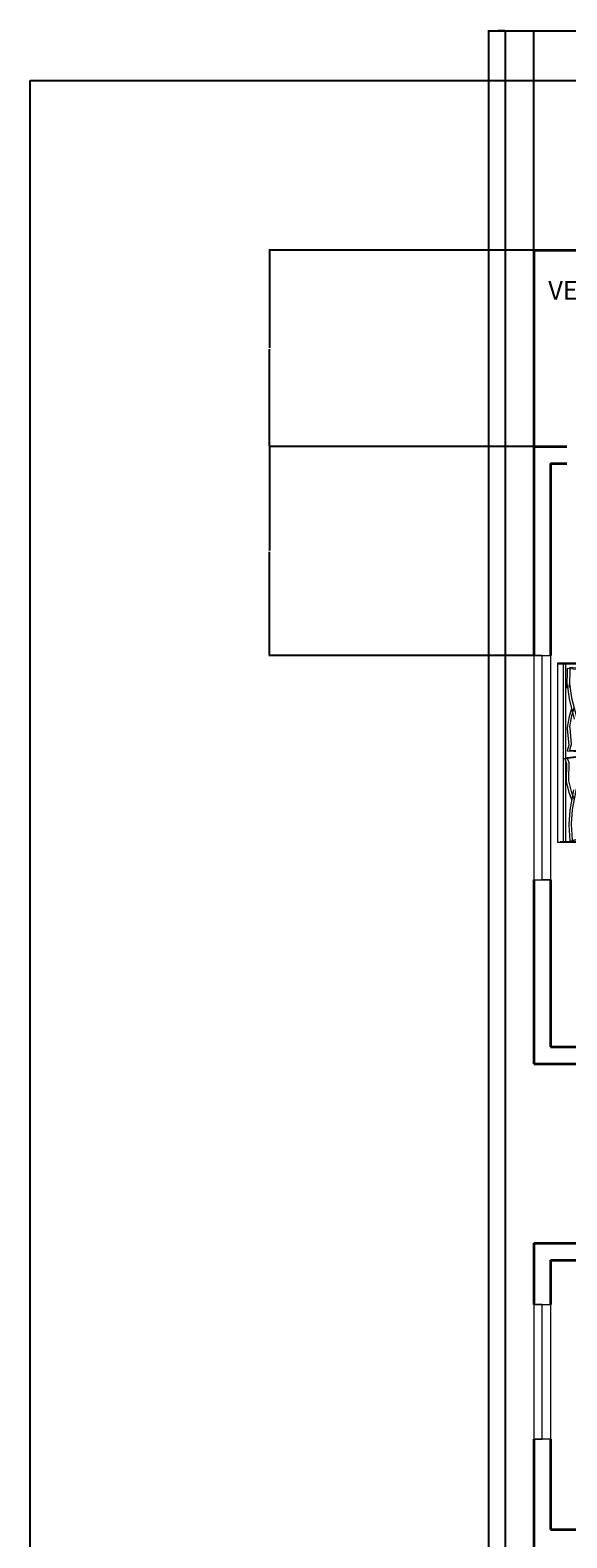
# Model space of a CAD drawing. Units: inches. Extents: x 2163 to 2982, y 1024 to 2288.
# Tile 10 of 22: x 2163 to 2306, y 1885 to 2288. Entities that reach past the tile are written whole.
import ezdxf

# ---------------------------------------------------------------- set-up
doc = ezdxf.new("R2010")
doc.units = ezdxf.units.IN
for name, color, linetype, lineweight in [('A-ANNO-DIMS', 2, 'Continuous', 18), ('A-ANNO-TTLB', 7, 'Continuous', 25), ('A-AREA-IDEN', 7, 'Continuous', 18), ('A-FURN', 8, 'Continuous', 13), ('A-GLAZ', 161, 'Continuous', 18), ('A-WALL', 7, 'Continuous', 35)]:
    doc.layers.add(name, color=color, linetype=linetype, lineweight=lineweight)
doc.styles.get("Standard").update_dxf_attribs({"font": 'arial.ttf'})
doc.dimstyles.get("Standard").update_dxf_attribs({"dimtxt": 0.18, "dimasz": 0.18, "dimexe": 0.18, "dimexo": 0.0625, "dimgap": 0.09, "dimtad": 0, "dimtih": 1, "dimtoh": 1, "dimdec": 4, "dimzin": 0, "dimdsep": 46, "dimtxsty": 'Standard', "dimcen": 0.09, "dimadec": 0, "dimazin": 0, "dimtfac": 1, "dimtdec": 4, "dimtofl": 0, "dimtmove": 0, "dimatfit": 3, "dimfxl": 1, "dimtolj": 1, "dimtzin": 0, "dimarcsym": 0})

# ---------------------------------------------------------------- blocks, each defined once
blk = doc.blocks.new('BED-DOUBLE')
for p, q in [((27.75, 52.87), (24.5, 49.16)), ((27.75, 52.87), (24.5, 49.16)), ((28.38, 53.1), (25.13, 49.39)), ((28.38, 53.1), (25.13, 49.39)), ((29.49, 52.95), (27.75, 52.87, 3.87)), ((29.49, 52.95), (27.75, 52.87, 3.87)), ((28.36, 51.33), (27.75, 52.87)), ((28.36, 51.33), (27.75, 52.87)), ((30.13, 53.18), (28.38, 53.1, 3.87)), ((29, 51.56), (28.38, 53.1)), ((30.13, 53.18), (28.38, 53.1, 3.87)), ((29, 51.56), (28.38, 53.1)), ((0, 51.49), (0.64, 51.49)), ((0, 3.47), (0, 51.49)), ((0, 51.27), (26.61, 51.27)), ((0, 51.27), (26.61, 51.27)), ((0.64, 51.49), (27.25, 51.49)), ((0.64, 51.49), (27.25, 51.49)), ((1.53, 3.48), (1.53, 51.27)), ((1.53, 3.47), (1.53, 51.27)), ((2.17, 3.7), (2.17, 51.49)), ((2.17, 3.7), (2.17, 51.49)), ((2.56, 50.11), (2.46, 44.71)), ((2.56, 50.11), (2.46, 44.71)), ((2.56, 50.11), (5.77, 49.73)), ((2.56, 50.11), (5.77, 49.73)), ((3.2, 50.34), (3.1, 44.94)), ((3.2, 50.34), (3.1, 44.94)), ((3.2, 50.34), (6.41, 49.96)), ((3.2, 50.34), (6.41, 49.96)), ((8.26, 49.31), (5.58, 48.13)), ((8.26, 49.31), (5.58, 48.13)), ((5.77, 49.73), (8.34, 50.33)), ((5.77, 49.73), (8.34, 50.33)), ((8.9, 49.54), (6.22, 48.36)), ((8.9, 49.54), (6.22, 48.36)), ((6.41, 49.96), (8.98, 50.56)), ((6.41, 49.96), (8.98, 50.56)), ((11.83, 50.11), (8.26, 49.31)), ((11.83, 50.11), (8.26, 49.31)), ((8.34, 50.33), (9.38, 49.81)), ((8.34, 50.33), (9.38, 49.81)), ((12.47, 50.34), (8.9, 49.54)), ((12.47, 50.34), (8.9, 49.54)), ((8.98, 50.56), (10.02, 50.04)), ((8.98, 50.56), (10.02, 50.04)), ((13.43, 49.92), (11.83, 50.11)), ((13.43, 49.92), (11.83, 50.11)), ((14.07, 50.15), (12.47, 50.34)), ((14.07, 50.15), (12.47, 50.34)), ((16.57, 50.7), (13.43, 49.92)), ((16.57, 50.7), (13.43, 49.92)), ((17.21, 50.93), (14.07, 50.15)), ((17.21, 50.93), (14.07, 50.15)), ((16.17, 45.57), (16.57, 50.7)), ((16.17, 45.57), (16.57, 50.7)), ((16.81, 45.79), (17.21, 50.93)), ((16.81, 45.79), (17.21, 50.93)), ((24.5, 49.16), (22.33, 46.22)), ((24.5, 49.16), (22.33, 46.22)), ((25.13, 49.39), (22.97, 46.45)), ((25.13, 49.39), (22.97, 46.45)), ((28.06, 48.23), (28.36, 51.33)), ((28.06, 48.23), (28.36, 51.33)), ((28.69, 48.46), (29, 51.56)), ((28.69, 48.46), (29, 51.56)), ((29, 44.59), (28.69, 48.46)), ((29, 44.59), (28.69, 48.46)), ((2.46, 44.71), (2.54, 45.71)), ((2.46, 44.71), (2.54, 45.71)), ((2.54, 45.71), (3.07, 41.91)), ((2.54, 45.71), (3.07, 41.91)), ((3.1, 44.94), (3.18, 45.94)), ((3.1, 44.94), (3.18, 45.94)), ((3.18, 45.94), (3.71, 42.14)), ((3.18, 45.94), (3.71, 42.14)), ((16.73, 43.61), (16.17, 45.57)), ((16.73, 43.61), (16.17, 45.57)), ((17.37, 43.83), (16.81, 45.79)), ((17.37, 43.83), (16.81, 45.79)), ((22.33, 46.22), (20.32, 40.64)), ((22.33, 46.22), (20.32, 40.64)), ((22.97, 46.45), (20.96, 40.87)), ((22.97, 46.45), (20.96, 40.87)), ((28.36, 44.36), (28.06, 48.23)), ((28.36, 44.36), (28.06, 48.23)), ((28.83, 40.95), (28.36, 44.36)), ((28.83, 40.95), (28.36, 44.36)), ((29.47, 41.18), (29, 44.59)), ((29.47, 41.18), (29, 44.59)), ((3.07, 41.91), (4.42, 36.49)), ((3.07, 41.91), (4.42, 36.49)), ((3.71, 42.14), (5.06, 36.72)), ((3.71, 42.14), (5.06, 36.72)), ((16.29, 36.6), (16.73, 43.61)), ((16.29, 36.6), (16.73, 43.61)), ((16.93, 36.82), (17.37, 43.83)), ((16.93, 36.82), (17.37, 43.83)), ((20.32, 40.64), (17.38, 32.31)), ((20.32, 40.64), (17.38, 32.31)), ((20.96, 40.87), (18.02, 32.53)), ((20.96, 40.87), (18.02, 32.53)), ((29.76, 38.94), (28.83, 40.95)), ((29.76, 38.94), (28.83, 40.95)), ((30.4, 39.17), (29.47, 41.18)), ((30.4, 39.17), (29.47, 41.18)), ((3.08, 37.14), (2.54, 34.2)), ((3.08, 37.13), (2.54, 34.2)), ((3.67, 39.2), (3.08, 37.14)), ((3.67, 39.2), (3.08, 37.13)), ((3.72, 37.36), (3.18, 34.43)), ((3.72, 37.36), (3.18, 34.43)), ((4.31, 39.43), (3.72, 37.36)), ((4.31, 39.43), (3.72, 37.36)), ((15.63, 32.56), (16.29, 36.6)), ((15.63, 32.56), (16.29, 36.6)), ((16.27, 32.79), (16.93, 36.82)), ((16.27, 32.79), (16.93, 36.82)), ((24.52, 34.68), (29, 36.38)), ((24.52, 34.68), (29, 36.38)), ((28.36, 36.15), (30.38, 36.46)), ((28.36, 36.15), (30.38, 36.46)), ((29, 36.38), (31.02, 36.69)), ((29, 36.38), (31.02, 36.69)), ((30.38, 36.46), (29.76, 38.94)), ((30.38, 36.46), (29.76, 38.94)), ((31.02, 36.69), (30.4, 39.17)), ((31.02, 36.69), (30.4, 39.17)), ((79.24, 15.06), (79.24, 39.68)), ((79.24, 15.06), (79.24, 39.68)), ((79.88, 15.29), (79.88, 39.91)), ((79.88, 15.29), (79.88, 39.91)), ((2.54, 34.2), (2.56, 33.88)), ((2.54, 34.2), (2.56, 33.88)), ((2.56, 33.88), (2.98, 29.46)), ((2.56, 33.88), (2.98, 29.46)), ((3.18, 34.43), (3.2, 34.11)), ((3.18, 34.43), (3.2, 34.11)), ((3.2, 34.11), (3.62, 29.68)), ((3.2, 34.11), (3.62, 29.68)), ((16.74, 30.75), (15.45, 33.82)), ((16.74, 30.75), (15.45, 33.82)), ((17.38, 30.98), (16.09, 34.05)), ((17.38, 30.98), (16.09, 34.05)), ((17.38, 30.26), (23.88, 34.45)), ((17.38, 30.26), (23.88, 34.45)), ((18.02, 30.49), (24.52, 34.68)), ((18.02, 30.49), (24.52, 34.68)), ((23.88, 34.45), (28.36, 36.15)), ((23.88, 34.45), (28.36, 36.15)), ((2.98, 29.46), (2.49, 27.98)), ((2.98, 29.46), (2.49, 27.98)), ((3.62, 29.68), (3.13, 28.21)), ((3.62, 29.68), (3.13, 28.2)), ((13.02, 27.66), (14.86, 28.36)), ((13.02, 27.66), (14.86, 28.36)), ((14.22, 28.13), (16.89, 28.3)), ((14.22, 28.13), (16.89, 28.3)), ((14.86, 28.36), (17.53, 28.53)), ((14.86, 28.36), (17.53, 28.53)), ((16.89, 28.3), (16.74, 30.75)), ((16.89, 28.3), (16.74, 30.75)), ((17.53, 28.53), (17.38, 30.98)), ((17.53, 28.53), (17.38, 30.98)), ((1.87, 25.98), (7.22, 26.56)), ((1.87, 25.98), (7.22, 26.56)), ((2.45, 24.54), (1.87, 25.98)), ((2.45, 24.54), (1.87, 25.98)), ((2.3, 20.09), (2.45, 24.54)), ((2.3, 20.09), (2.45, 24.54)), ((2.49, 27.98), (7.87, 27.73)), ((2.49, 27.98), (7.87, 27.73)), ((2.51, 26.21), (7.86, 26.79)), ((2.51, 26.21), (7.86, 26.79)), ((3.09, 24.77), (2.51, 26.21)), ((3.09, 24.77), (2.51, 26.21)), ((2.94, 20.32), (3.09, 24.77)), ((2.94, 20.32), (3.09, 24.77)), ((3.13, 28.21), (8.51, 27.96)), ((3.13, 28.2), (8.51, 27.96)), ((7.22, 26.56), (10.4, 27.14)), ((7.22, 26.56), (10.4, 27.14)), ((7.86, 26.79), (11.04, 27.37)), ((7.86, 26.79), (11.04, 27.37)), ((7.87, 27.73), (11.08, 27.35)), ((7.87, 27.73), (11.08, 27.35)), ((8.51, 27.96), (11.72, 27.58)), ((8.51, 27.96), (11.72, 27.58)), ((10.4, 27.14), (11.7, 27.14)), ((10.4, 27.14), (11.7, 27.14)), ((11.04, 27.37), (12.34, 27.37)), ((11.04, 27.37), (12.34, 27.37)), ((11.08, 27.35), (12.38, 27.44)), ((11.08, 27.35), (12.38, 27.44)), ((11.7, 27.14), (13.58, 26.56)), ((11.7, 27.14), (13.58, 26.56)), ((11.72, 27.58), (13.02, 27.66)), ((11.72, 27.58), (13.02, 27.66)), ((12.34, 27.37), (14.22, 26.79)), ((12.34, 27.37), (14.22, 26.79)), ((12.38, 27.44), (14.22, 28.13)), ((12.38, 27.44), (14.22, 28.13)), ((13.58, 26.56), (16.26, 26.56)), ((13.58, 26.56), (16.26, 26.56)), ((14.22, 26.79), (16.9, 26.79)), ((14.22, 26.79), (16.9, 26.79)), ((16.9, 24.33), (15.81, 21.19)), ((16.9, 24.33), (15.81, 21.19)), ((16.17, 19.38), (16.57, 24.52)), ((16.17, 19.38), (16.57, 24.52)), ((16.26, 26.56), (16.26, 24.1)), ((16.26, 26.56), (16.26, 24.1)), ((16.81, 19.61), (17.21, 24.74)), ((16.81, 19.61), (17.21, 24.74)), ((16.9, 26.79), (16.9, 24.33)), ((16.9, 26.79), (16.9, 24.33)), ((2.94, 20), (2.94, 20.32)), ((2.94, 20), (2.94, 20.32)), ((16.26, 24.1), (15.17, 20.96)), ((16.26, 24.1), (15.17, 20.96)), ((2.3, 19.77), (2.3, 20.09)), ((2.3, 19.77), (2.3, 20.09)), ((3.03, 16.88), (2.3, 19.77)), ((3.03, 16.88), (2.3, 19.77)), ((3.67, 17.11), (2.94, 20)), ((3.67, 17.11), (2.94, 20)), ((3.75, 14.85), (3.03, 16.88)), ((3.75, 14.85), (3.03, 16.88)), ((3.32, 12.11), (4.33, 17.6)), ((3.32, 12.11), (4.33, 17.6)), ((4.39, 15.08), (3.67, 17.11)), ((4.39, 15.08), (3.67, 17.11)), ((3.96, 12.34), (4.97, 17.83)), ((3.96, 12.34), (4.97, 17.83)), ((16.73, 17.42), (16.17, 19.38)), ((16.73, 17.42), (16.17, 19.38)), ((16.29, 10.41), (16.73, 17.42)), ((16.29, 10.41), (16.73, 17.42)), ((17.37, 17.65), (16.81, 19.61)), ((17.37, 17.65), (16.81, 19.61)), ((16.93, 10.64), (17.37, 17.65)), ((16.93, 10.64), (17.37, 17.65)), ((3.03, 8.28), (3.32, 12.11)), ((3.03, 8.28), (3.32, 12.11)), ((3.67, 8.51), (3.96, 12.34)), ((3.67, 8.51), (3.96, 12.34)), ((3.01, 8.18), (3.03, 8.28)), ((3.01, 8.18), (3.03, 8.28)), ((3.34, 3.9), (3.01, 8.18)), ((3.34, 3.9), (3.01, 8.18)), ((3.65, 8.41), (3.67, 8.51)), ((3.65, 8.41), (3.67, 8.51)), ((3.98, 4.13), (3.65, 8.41)), ((3.98, 4.13), (3.65, 8.41)), ((15.63, 6.38), (16.29, 10.41)), ((15.63, 6.38), (16.29, 10.41)), ((16.27, 6.61), (16.93, 10.64)), ((16.27, 6.61), (16.93, 10.64)), ((16.29, 10.41), (16.62, 9.28)), ((16.29, 10.41), (16.62, 9.28)), ((16.62, 9.28), (17.34, 4.18)), ((16.62, 9.28), (17.34, 4.18)), ((16.93, 10.64), (17.26, 9.51)), ((16.93, 10.64), (17.26, 9.51)), ((17.26, 9.51), (17.98, 4.41)), ((17.26, 9.51), (17.98, 4.41)), ((3.32, 3.89), (6.5, 4.47)), ((3.32, 3.89), (6.5, 4.47)), ((3.96, 4.12), (7.14, 4.7)), ((3.96, 4.12), (7.14, 4.7)), ((8.95, 5.05), (6.21, 6.06)), ((8.95, 5.05), (6.21, 6.06)), ((6.5, 4.47), (9.1, 4.04)), ((6.5, 4.47), (9.1, 4.04)), ((9.59, 5.28), (6.85, 6.29)), ((9.59, 5.28), (6.85, 6.29)), ((7.14, 4.7), (9.74, 4.27)), ((7.14, 4.7), (9.74, 4.27)), ((12.57, 4.47), (8.95, 5.05)), ((12.57, 4.47), (8.95, 5.05)), ((9.1, 4.04), (10.11, 4.62)), ((9.1, 4.04), (10.11, 4.62)), ((13.21, 4.7), (9.59, 5.28)), ((13.21, 4.7), (9.59, 5.28)), ((9.74, 4.27), (10.75, 4.85)), ((9.74, 4.27), (10.75, 4.85)), ((14.16, 4.76), (12.57, 4.47)), ((14.16, 4.76), (12.57, 4.47)), ((14.8, 4.99), (13.21, 4.7)), ((14.8, 4.99), (13.21, 4.7)), ((17.34, 4.18), (14.16, 4.76)), ((17.34, 4.18), (14.16, 4.76)), ((17.98, 4.41), (14.8, 4.99)), ((17.98, 4.41), (14.8, 4.99)), ((18.11, 3.48), (0, 3.48)), ((18.11, 3.47), (0, 3.47)), ((18.75, 3.7), (0.64, 3.7)), ((18.75, 3.7), (0.64, 3.7))]:
    blk.add_line(p, q)
for centre, radius, start, end in [((-6.66, 51.33), 36.18, 349.8763, 2.5657), ((-6.66, 51.33), 36.18, 349.8763, 2.5657), ((36.31, 182.27), 129.5, 266.9791, 273.8365), ((36.31, 182.27), 129.5, 266.9791, 273.8365), ((-6.02, 51.56), 36.18, 349.8763, 2.5657), ((-6.02, 51.56), 36.18, 349.8763, 2.5657), ((36.95, 182.49), 129.5, 266.9791, 273.8365), ((36.95, 182.49), 129.5, 266.9791, 273.8365), ((67.82, -4508.74), 4561.86, 90.00217, 90.28689), ((67.82, -4508.74), 4561.86, 90.00217, 90.28689), ((68.46, -4508.52), 4561.86, 90.00217, 90.28689), ((68.46, -4508.52), 4561.86, 90.00217, 90.28689), ((68.67, 76.16), 23.07, 267.4714, 296.4681), ((68.67, 76.16), 23.07, 267.4714, 296.4681), ((69.31, 76.39), 23.07, 267.4714, 296.4681), ((69.31, 76.39), 23.07, 267.4714, 296.4681), ((78.87, 54.41), 1.1, 332.6588, 86.02), ((78.87, 54.41), 1.1, 332.6588, 86.02), ((212.28, 41.15), 133.04, 174.4998, 180.6351), ((212.28, 41.15), 133.04, 174.4998, 180.6351), ((79.51, 54.64), 1.1, 332.6588, 86.02), ((79.51, 54.64), 1.1, 332.6588, 86.02), ((212.92, 41.38), 133.04, 174.4998, 180.6351), ((212.92, 41.38), 133.04, 174.4998, 180.6351), ((35.07, 43.74), 6.22, 168.6608, 203.7384), ((35.07, 43.74), 6.22, 168.6608, 203.7384), ((35.71, 43.97), 6.22, 168.6608, 203.7384), ((35.71, 43.97), 6.22, 168.6608, 203.7384), ((1.48, 31.15), 29.65, 10.6617, 19.8806), ((1.48, 31.15), 29.65, 10.6617, 19.8806), ((2.12, 31.38), 29.65, 10.6617, 19.8806), ((2.12, 31.38), 29.65, 10.6617, 19.8806), ((156.96, 17.98), 129.02, 171.7845, 186.9006), ((156.96, 17.98), 129.02, 171.7845, 186.9006), ((30.44, 36.64), 0.185, 250.2464, 1.1377), ((30.44, 36.64), 0.185, 250.2464, 1.1377), ((31.08, 36.86), 0.185, 250.2464, 1.1377), ((31.08, 36.86), 0.185, 250.2464, 1.1377), ((182.05, 21.36), 164.97, 176.0865, 186.7821), ((182.05, 21.36), 164.97, 176.0865, 186.7821), ((182.69, 21.59), 164.97, 176.0865, 186.7821), ((182.69, 21.59), 164.97, 176.0865, 186.7821), ((156.32, 17.76), 129.02, 171.7845, 186.9006), ((156.32, 17.76), 129.02, 171.7845, 186.9006), ((-23.71, -17.22), 106.46, 13.3832, 17.7053), ((-23.71, -17.22), 106.46, 13.3832, 17.7053), ((-23.07, -16.99), 106.46, 13.3832, 17.7053), ((-23.07, -16.99), 106.46, 13.3832, 17.7053), ((200.84, 21.43), 121.76, 182.9958, 189.4091), ((200.84, 21.43), 121.76, 182.9958, 189.4091), ((201.48, 21.66), 121.76, 182.9958, 189.4091), ((201.48, 21.65), 121.76, 182.9958, 189.4091), ((20.1, 85.16), 83.31, 268.7218, 275.604), ((20.1, 85.16), 83.31, 268.7218, 275.604), ((20.74, 85.39), 83.31, 268.7218, 275.604), ((20.74, 85.39), 83.31, 268.7218, 275.604), ((31.17, -167.31), 170.11, 88.4762, 91.0082), ((31.17, -167.31), 170.11, 88.4762, 91.0082), ((31.81, -167.08), 170.11, 88.4762, 91.0082), ((31.81, -167.08), 170.11, 88.4762, 91.0082), ((50.61, 484.82), 482.31, 268.2277, 271.7185), ((50.61, 484.82), 482.31, 268.2277, 271.7185), ((51.25, 485.05), 482.31, 268.2277, 271.7185), ((51.25, 485.05), 482.31, 268.2277, 271.7185), ((64.51, -26.9), 29.63, 76.0648, 88.9113), ((64.51, -26.9), 29.63, 76.0648, 88.9113), ((65.15, -26.67), 29.63, 76.0648, 88.9113), ((65.15, -26.67), 29.63, 76.0648, 88.9113), ((70.28, -21.66), 23.56, 67.9751, 86.652), ((70.28, -21.66), 23.56, 67.9751, 86.652), ((70.91, -21.43), 23.56, 67.9751, 86.652), ((70.91, -21.43), 23.56, 67.9751, 86.652), ((79.72, 1.09), 1.09, 236.1736, 23.4781), ((79.72, 1.09), 1.09, 236.1736, 23.4781), ((80.36, 1.32), 1.09, 236.1736, 23.4781), ((80.36, 1.32), 1.09, 236.1736, 23.4781)]:
    blk.add_arc(centre, radius, start, end)
blk = doc.blocks.new('WIN-60')
for p, q in [((2.25, 60), (0, 60)), ((0, 60), (4.5, 60)), ((0, 60), (0, 0)), ((2.25, 0), (2.25, 60)), ((4.5, 60), (4.5, 0)), ((0, 0), (4.5, 0)), ((4.5, 0), (2.25, 0))]:
    blk.add_line(p, q)
blk = doc.blocks.new('WIN-36-ALT')
for p, q in [((2.25, 36), (0, 36)), ((0, 36), (4.5, 36)), ((0, 36), (0, 0)), ((2.25, 0), (2.25, 36)), ((4.5, 36), (4.5, 0)), ((4.5, 0), (0, 0)), ((0, 0), (2.25, 0))]:
    blk.add_line(p, q)
blk = doc.blocks.new('*D27')
at = {"layer": 'A-ANNO-DIMS', "color": 0, "lineweight": -2, "transparency": 16777216}
for p, q in [((2297.28, 2176.77), (2226.51, 2176.77)), ((2226.69, 2176.59), (2226.69, 2149.02)), ((2226.69, 2121.1), (2226.69, 2148.66)), ((2297.28, 2120.92), (2226.51, 2120.92))]:
    blk.add_line(p, q, dxfattribs=at)
at = {"layer": 'A-ANNO-DIMS', "color": 0, "transparency": 16777216}
for points in [[(2226.66, 2176.59), (2226.72, 2176.59), (2226.69, 2176.77)], [(2226.66, 2121.1), (2226.72, 2121.1), (2226.69, 2120.92)]]:
    blk.add_solid(points, dxfattribs=at)
at = {"layer": 'Defpoints', "color": 0, "transparency": 16777216}
for p in [(2297.34, 2176.77), (2226.69, 2120.92), (2297.34, 2120.92)]:
    blk.add_point(p, dxfattribs=at)
at = {"layer": 'A-ANNO-DIMS', "color": 0, "transparency": 16777216, "insert": (2226.69, 2148.84), "char_height": 0.18, "attachment_point": 5}
blk.add_mtext('\\A1;55.85', dxfattribs=at)
blk = doc.blocks.new('*D28')
at = {"layer": 'A-ANNO-DIMS', "color": 0, "lineweight": -2, "transparency": 16777216}
for p, q in [((2297.34, 2229.33), (2297.34, 2288.1)), ((2297.52, 2287.92), (2439.55, 2287.92)), ((2582.16, 2287.92), (2440.13, 2287.92)), ((2582.34, 2229.33), (2582.34, 2288.1))]:
    blk.add_line(p, q, dxfattribs=at)
at = {"layer": 'A-ANNO-DIMS', "color": 0, "transparency": 16777216}
for points in [[(2297.52, 2287.95), (2297.52, 2287.89), (2297.34, 2287.92)], [(2582.16, 2287.95), (2582.16, 2287.89), (2582.34, 2287.92)]]:
    blk.add_solid(points, dxfattribs=at)
at = {"layer": 'Defpoints', "color": 0, "transparency": 16777216}
for p in [(2582.34, 2287.92), (2297.34, 2229.27), (2582.34, 2229.27)]:
    blk.add_point(p, dxfattribs=at)
at = {"layer": 'A-ANNO-DIMS', "color": 0, "transparency": 16777216, "insert": (2439.84, 2287.92), "char_height": 0.18, "attachment_point": 5}
blk.add_mtext('\\A1;285', dxfattribs=at)
blk = doc.blocks.new('*D29')
at = {"layer": 'A-ANNO-DIMS', "color": 0, "lineweight": -2, "transparency": 16777216}
for p, q in [((2285.34, 1738.83), (2285.34, 2288.1)), ((2285.52, 2287.92), (2576.05, 2287.92)), ((2867.16, 2287.92), (2576.63, 2287.92)), ((2867.34, 2229.33), (2867.34, 2288.1))]:
    blk.add_line(p, q, dxfattribs=at)
at = {"layer": 'A-ANNO-DIMS', "color": 0, "transparency": 16777216}
for points in [[(2285.52, 2287.95), (2285.52, 2287.89), (2285.34, 2287.92)], [(2867.16, 2287.95), (2867.16, 2287.89), (2867.34, 2287.92)]]:
    blk.add_solid(points, dxfattribs=at)
at = {"layer": 'Defpoints', "color": 0, "transparency": 16777216}
for p in [(2867.34, 2287.92), (2867.34, 2229.27), (2285.34, 1738.77)]:
    blk.add_point(p, dxfattribs=at)
at = {"layer": 'A-ANNO-DIMS', "color": 0, "transparency": 16777216, "insert": (2576.34, 2287.92), "char_height": 0.18, "attachment_point": 5}
blk.add_mtext('\\A1;582', dxfattribs=at)
blk = doc.blocks.new('*D35')
at = {"layer": 'A-ANNO-DIMS', "color": 0, "lineweight": -2, "transparency": 16777216}
for p, q in [((2297.28, 2229.27), (2226.51, 2229.27)), ((2226.69, 2229.09), (2226.69, 2203.2)), ((2226.69, 2176.95), (2226.69, 2202.84)), ((2297.28, 2176.77), (2226.51, 2176.77))]:
    blk.add_line(p, q, dxfattribs=at)
at = {"layer": 'A-ANNO-DIMS', "color": 0, "transparency": 16777216}
for points in [[(2226.66, 2229.09), (2226.72, 2229.09), (2226.69, 2229.27)], [(2226.66, 2176.95), (2226.72, 2176.95), (2226.69, 2176.77)]]:
    blk.add_solid(points, dxfattribs=at)
at = {"layer": 'Defpoints', "color": 0, "transparency": 16777216}
for p in [(2297.34, 2229.27), (2226.69, 2176.77), (2297.34, 2176.77)]:
    blk.add_point(p, dxfattribs=at)
at = {"layer": 'A-ANNO-DIMS', "color": 0, "transparency": 16777216, "insert": (2226.69, 2203.02), "char_height": 0.18, "attachment_point": 5}
blk.add_mtext('\\A1;52.5', dxfattribs=at)
blk = doc.blocks.new('*D40')
at = {"layer": 'A-ANNO-DIMS', "color": 0, "lineweight": -2, "transparency": 16777216}
for p, q in [((2285.34, 1738.83), (2285.34, 2288.1)), ((2285.52, 2287.92), (2287.33, 2287.92)), ((2289.66, 2287.92), (2287.85, 2287.92)), ((2289.84, 1734.33), (2289.84, 2288.1))]:
    blk.add_line(p, q, dxfattribs=at)
at = {"layer": 'A-ANNO-DIMS', "color": 0, "transparency": 16777216}
for points in [[(2285.52, 2287.95), (2285.52, 2287.89), (2285.34, 2287.92)], [(2289.66, 2287.95), (2289.66, 2287.89), (2289.84, 2287.92)]]:
    blk.add_solid(points, dxfattribs=at)
at = {"layer": 'Defpoints', "color": 0, "transparency": 16777216}
for p in [(2289.84, 2287.92), (2285.34, 1738.77), (2289.84, 1734.27)]:
    blk.add_point(p, dxfattribs=at)
at = {"layer": 'A-ANNO-DIMS', "color": 0, "transparency": 16777216, "insert": (2287.59, 2287.92), "char_height": 0.18, "attachment_point": 5}
blk.add_mtext('\\A1;4.5', dxfattribs=at)

msp = doc.modelspace()

# ---------------------------------------------------------------- linework, layer by layer
at = {"layer": 'A-ANNO-TTLB'}
msp.add_lwpolyline([(2162.6841, 2274.6054), (2982.469, 2274.6054), (2982.469, 1045.9691), (2162.6841, 1045.9691)], close=True, dxfattribs=at)
at = {"layer": 'A-WALL'}
for p, q in [((2297.3389, 2229.2688), (2414.7613, 2229.2688)), ((2297.3389, 2229.2688), (2297.3389, 2120.915)), ((2297.3389, 2176.7688), (2306.2073, 2176.7688)), ((2301.8389, 2172.2688), (2306.2073, 2172.2688)), ((2301.8389, 2172.2688), (2301.8389, 2120.915)), ((2297.3389, 2060.915), (2297.3389, 2011.7688)), ((2301.8389, 2060.915), (2301.8389, 2016.2688)), ((2301.8389, 2016.2688), (2417.447, 2016.2688)), ((2297.3389, 2011.7688), (2321.3389, 2011.7688)), ((2297.3389, 1963.7688), (2321.3389, 1963.7688)), ((2297.3389, 1963.7688), (2297.3389, 1947.3655)), ((2301.8389, 1959.2688), (2422.6267, 1959.2688)), ((2301.8389, 1959.2688), (2301.8389, 1947.3655)), ((2297.3389, 1911.3655), (2297.3389, 1828.6523)), ((2301.8389, 1911.3655), (2301.8389, 1887.2688)), ((2301.8389, 1887.2688), (2445.8389, 1887.2688))]:
    msp.add_line(p, q, dxfattribs=at)

# ---------------------------------------------------------------- block references
at = {"layer": 'A-FURN'}
msp.add_blockref('BED-DOUBLE', (2303.774, 2067.438), dxfattribs=at)
at = {"layer": 'A-GLAZ'}
for name, p in [('WIN-60', (2297.339, 2060.915)), ('WIN-36-ALT', (2297.339, 1911.366))]:
    msp.add_blockref(name, p, dxfattribs=at)

# ---------------------------------------------------------------- texts
at = {"layer": 'A-AREA-IDEN', "insert": (2301.2277, 2221.0494), "char_height": 5, "attachment_point": 1}
msp.add_mtext_dynamic_manual_height_columns('VERANDA', width=48.491843, gutter_width=12.5, heights=[0], dxfattribs=at)

# ---------------------------------------------------------------- dimensions: what is measured, and where the dimension line sits
at = {"layer": 'A-ANNO-DIMS'}
for base, p1, p2, override, picture, middle in [((2867.3389, 2287.9188), (2285.3389, 1738.7688), (2867.3389, 2229.2688), {"dimdec": 0, "dimlfac": 1, "dimrnd": 0, "dimzin": 0, "dimdsep": 46, "dimlunit": 2}, '*D29', (2576.3389, 2287.9188)), ((2289.8389, 2287.9188), (2285.3389, 1738.7688), (2289.8389, 1734.2688), {"dimdec": 1, "dimlfac": 1, "dimrnd": 0, "dimzin": 0, "dimdsep": 46, "dimlunit": 2}, '*D40', (2287.5889, 2287.9188)), ((2582.3389, 2287.9188), (2297.3389, 2229.2688), (2582.3389, 2229.2688), {"dimdec": 0, "dimlfac": 1, "dimrnd": 0, "dimzin": 0, "dimdsep": 46, "dimlunit": 2}, '*D28', (2439.8389, 2287.9188))]:
    dim = msp.add_linear_dim(base=base, p1=p1, p2=p2, dimstyle='Standard', override=override, dxfattribs=at)
    dim.commit()
    dim.dimension.update_dxf_attribs({"geometry": picture, "text_midpoint": middle})
for base, p1, p2, override, picture, middle in [((2226.6889, 2176.7688), (2297.3389, 2229.2688), (2297.3389, 2176.7688), {"dimdec": 1, "dimlfac": 1, "dimrnd": 0, "dimzin": 0, "dimdsep": 46, "dimlunit": 2}, '*D35', (2226.6889, 2203.0188)), ((2226.6889, 2120.915), (2297.3389, 2176.7688), (2297.3389, 2120.915), {"dimdec": 2, "dimlfac": 1, "dimrnd": 0, "dimzin": 0, "dimdsep": 46, "dimlunit": 2}, '*D27', (2226.6889, 2148.8419))]:
    dim = msp.add_linear_dim(base=base, p1=p1, p2=p2, angle=90, dimstyle='Standard', override=override, dxfattribs=at)
    dim.commit()
    dim.dimension.update_dxf_attribs({"geometry": picture, "text_midpoint": middle})

doc.saveas('drawing.dxf')
